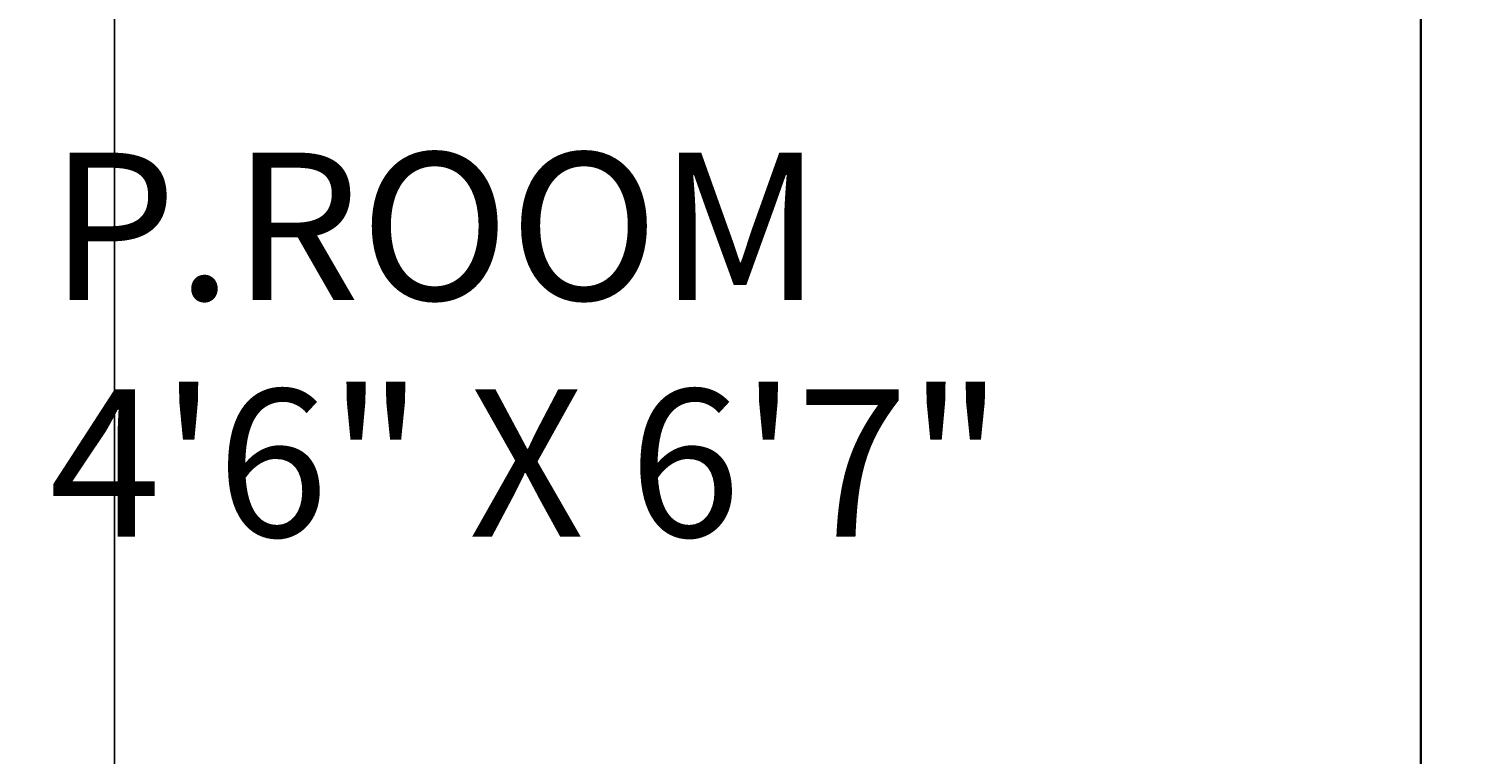
# Model space of a CAD drawing. Units: inches. Extents: x -61 to 1599, y -1316 to 257.
# Tile 87 of 204: x 274 to 321, y -342 to -318. Entities that reach past the tile are written whole.
import ezdxf

# ---------------------------------------------------------------- set-up
doc = ezdxf.new("R2010")
doc.units = ezdxf.units.IN
doc.header["$MEASUREMENT"] = 0
for name, color, linetype, lineweight in [('A-ANNO-DIMS', 2, 'Continuous', 18), ('A-AREA-IDEN', 1, 'Continuous', 18), ('WALLS', 4, 'Continuous', 35)]:
    doc.layers.add(name, color=color, linetype=linetype, lineweight=lineweight)
doc.styles.get("Standard").update_dxf_attribs({"font": 'arial.ttf'})
doc.dimstyles.get("Standard").update_dxf_attribs({"dimtxt": 0.18, "dimasz": 0.18, "dimexe": 0.18, "dimexo": 0.0625, "dimgap": 0.09, "dimtad": 0, "dimtih": 1, "dimtoh": 1, "dimdec": 0, "dimzin": 0, "dimdsep": 46, "dimlunit": 3, "dimtxsty": 'Standard', "dimcen": 0.09, "dimadec": 0, "dimazin": 0, "dimtfac": 1, "dimtdec": 0, "dimtofl": 0, "dimtmove": 0, "dimatfit": 3, "dimfxl": 1, "dimtolj": 1, "dimtzin": 0, "dimarcsym": 0})

# ---------------------------------------------------------------- blocks, each defined once
blk = doc.blocks.new('*D687')
at = {"layer": 'A-ANNO-DIMS', "color": 0, "lineweight": -2, "transparency": 16777216}
for p, q in [((289.418, 181.677), (-61.077, 181.677)), ((-60.897, 181.497), (-60.897, -528.952)), ((-60.897, -1239.765), (-60.897, -529.316)), ((319.64, -1239.945), (-61.077, -1239.945))]:
    blk.add_line(p, q, dxfattribs=at)
at = {"layer": 'A-ANNO-DIMS', "color": 0, "transparency": 16777216}
for points in [[(-60.927, 181.497), (-60.867, 181.497), (-60.897, 181.677)], [(-60.927, -1239.765), (-60.867, -1239.765), (-60.897, -1239.945)]]:
    blk.add_solid(points, dxfattribs=at)
at = {"layer": 'DEFPOINTS', "color": 0, "transparency": 16777216}
for p in [(289.481, 181.677), (-60.897, -1239.945), (319.703, -1239.945)]:
    blk.add_point(p, dxfattribs=at)
at = {"layer": 'A-ANNO-DIMS', "color": 0, "transparency": 16777216, "insert": (-60.897, -529.134), "char_height": 0.18, "attachment_point": 5}
blk.add_mtext('\\A1;1421.6', dxfattribs=at)
blk = doc.blocks.new('*D699')
at = {"layer": 'A-ANNO-DIMS', "color": 0, "lineweight": -2, "transparency": 16777216}
for p, q in [((835.64, -167.169), (-61.077, -167.169)), ((-60.897, -167.349), (-60.897, -306.726)), ((-60.897, -446.466), (-60.897, -307.09)), ((841.64, -446.646), (-61.077, -446.646))]:
    blk.add_line(p, q, dxfattribs=at)
at = {"layer": 'A-ANNO-DIMS', "color": 0, "transparency": 16777216}
for points in [[(-60.927, -167.349), (-60.867, -167.349), (-60.897, -167.169)], [(-60.927, -446.466), (-60.867, -446.466), (-60.897, -446.646)]]:
    blk.add_solid(points, dxfattribs=at)
at = {"layer": 'DEFPOINTS', "color": 0, "transparency": 16777216}
for p in [(835.703, -167.169), (-60.897, -446.646), (841.703, -446.646)]:
    blk.add_point(p, dxfattribs=at)
at = {"layer": 'A-ANNO-DIMS', "color": 0, "transparency": 16777216, "insert": (-60.897, -306.908), "char_height": 0.18, "attachment_point": 5}
blk.add_mtext('\\A1;279.5', dxfattribs=at)
blk = doc.blocks.new('*D702')
at = {"layer": 'A-ANNO-DIMS', "color": 0, "lineweight": -2, "transparency": 16777216}
for p, q in [((276.882, -616.882), (276.882, 257.457)), ((277.062, 257.277), (312.209, 257.277)), ((348.14, 257.277), (312.994, 257.277)), ((348.32, -616.882), (348.32, 257.457))]:
    blk.add_line(p, q, dxfattribs=at)
at = {"layer": 'A-ANNO-DIMS', "color": 0, "transparency": 16777216}
for points in [[(277.062, 257.307), (277.062, 257.247), (276.882, 257.277)], [(348.14, 257.307), (348.14, 257.247), (348.32, 257.277)]]:
    blk.add_solid(points, dxfattribs=at)
at = {"layer": 'DEFPOINTS', "color": 0, "transparency": 16777216}
for p in [(348.32, 257.277), (276.882, -616.945), (348.32, -616.945)]:
    blk.add_point(p, dxfattribs=at)
at = {"layer": 'A-ANNO-DIMS', "color": 0, "transparency": 16777216, "insert": (312.601, 257.277), "char_height": 0.18, "attachment_point": 5}
blk.add_mtext('\\A1;71.44', dxfattribs=at)

msp = doc.modelspace()

# ---------------------------------------------------------------- linework, layer by layer
at = {"layer": 'WALLS'}
msp.add_line((319.7028, -288.3229), (319.7028, -367.3229), dxfattribs=at)

# ---------------------------------------------------------------- texts
at = {"layer": 'A-AREA-IDEN'}
for s, height, p in [('P.ROOM', 4.8321, (274.7407, -326.9772)), ('4\'6" X 6\'7"', 4.832098, (274.7407, -334.7395))]:
    msp.add_text(s, height=height, dxfattribs=at).set_placement(p)

# ---------------------------------------------------------------- dimensions: what is measured, and where the dimension line sits
at = {"layer": 'A-ANNO-DIMS'}
dim = msp.add_linear_dim(base=(348.3201, 257.2771), p1=(276.8825, -616.9446), p2=(348.3201, -616.9446), dimstyle='Standard', override={"dimdec": 2, "dimlfac": 1, "dimrnd": 0, "dimzin": 0, "dimdsep": 46, "dimlunit": 2}, dxfattribs=at)
dim.commit()
dim.dimension.update_dxf_attribs({"geometry": '*D702', "text_midpoint": (312.6013, 257.2771)})
for base, p1, p2, picture, middle in [((-60.8972, -1239.9446), (289.4807, 181.6771), (319.7028, -1239.9446), '*D687', (-60.8972, -529.1337)), ((-60.8972, -446.6462), (835.7028, -167.169), (841.7028, -446.6462), '*D699', (-60.8972, -306.9076))]:
    dim = msp.add_linear_dim(base=base, p1=p1, p2=p2, angle=90, dimstyle='Standard', override={"dimdec": 1, "dimlfac": 1, "dimrnd": 0, "dimzin": 0, "dimdsep": 46, "dimlunit": 2}, dxfattribs=at)
    dim.commit()
    dim.dimension.update_dxf_attribs({"geometry": picture, "text_midpoint": middle})

doc.saveas('drawing.dxf')
